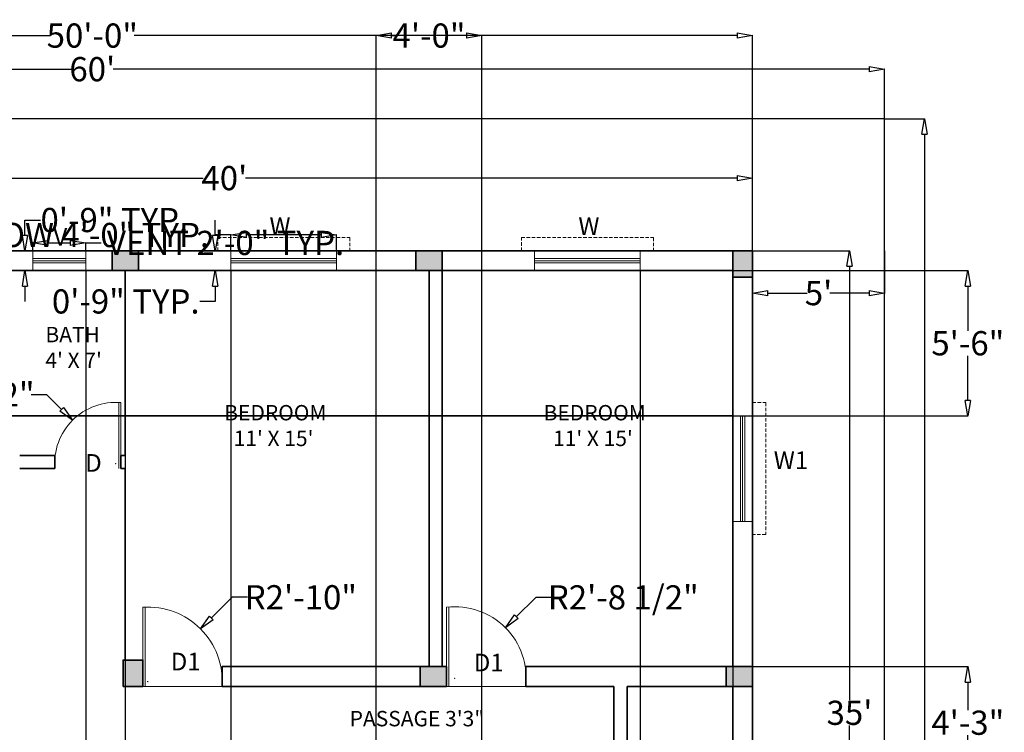
# Model space of a CAD drawing. Units: inches. Extents: x 668 to 1552, y 994 to 1684.
# Tile 4 of 4: x 1061 to 1509, y 1360 to 1684. Entities that reach past the tile are written whole.
import ezdxf

# ---------------------------------------------------------------- set-up
doc = ezdxf.new("R2010")
doc.units = ezdxf.units.IN
doc.header["$LTSCALE"] = 2.5
doc.header["$MEASUREMENT"] = 0
doc.linetypes.add('HIDDEN', pattern=[0.375, 0.25, -0.125])
for name, color, linetype, lineweight, true_color in [('A-ANNO-DIMS', 175, 'Continuous', 13, 0x4554a5), ('A-ANNO-TEXT', 52, 'Continuous', 18, 0xc8c92d), ('A-DOOR', 152, 'Continuous', 18, 0x2776bb)]:
    doc.layers.add(name, color=color, linetype=linetype, lineweight=lineweight, true_color=true_color)
for name, color, linetype, lineweight in [('A-AREA-IDEN', 2, 'Continuous', 18), ('A-COLS', 7, 'Continuous', 35), ('A-COLS-PATT', 1, 'Continuous', 13), ('A-GLAZ', 4, 'Continuous', 18), ('A-WALL', 7, 'Continuous', 35), ('C-PROP', 1, 'Continuous', 25), ('sajjas', 210, 'HIDDEN', 13)]:
    doc.layers.add(name, color=color, linetype=linetype, lineweight=lineweight)
doc.styles.get("Standard").update_dxf_attribs({"font": 'arial.ttf'})
doc.dimstyles.get("Standard").update_dxf_attribs({"dimtxt": 11, "dimasz": 7, "dimexe": 0.18, "dimexo": 0.0625, "dimgap": 0.09, "dimtad": 0, "dimtih": 1, "dimtoh": 1, "dimdec": 0, "dimzin": 0, "dimdsep": 46, "dimlunit": 3, "dimtxsty": 'Standard', "dimblk": 'CLOSEDBLANK', "dimcen": 0.09, "dimadec": 0, "dimazin": 0, "dimtfac": 1, "dimtdec": 0, "dimtofl": 0, "dimtmove": 0, "dimatfit": 3, "dimldrblk": 'CLOSEDBLANK', "dimfxl": 1, "dimtolj": 1, "dimtzin": 0, "dimarcsym": 0})

# ---------------------------------------------------------------- blocks, each defined once
blk = doc.blocks.new('_ClosedBlank')
at = {"color": 0, "linetype": 'ByBlock', "lineweight": -2}
for p, q in [((-1, 0.167), (0, 0)), ((-1, 0.167), (-1, -0.167)), ((0, 0), (-1, -0.167))]:
    blk.add_line(p, q, dxfattribs=at)
blk = doc.blocks.new('*D1')
at = {"layer": 'A-ANNO-DIMS', "color": 0, "lineweight": -2, "ltscale": 2.5, "transparency": 16777216}
for p, q in [((734.36, 1639.41), (734.36, 1662.1)), ((741.36, 1661.92), (1084.91, 1661.92)), ((1447.36, 1661.92), (1103.82, 1661.92)), ((1454.36, 1639.41), (1454.36, 1662.1))]:
    blk.add_line(p, q, dxfattribs=at)
at = {"layer": 'Defpoints', "color": 0, "ltscale": 2.5, "transparency": 16777216}
for p in [(1454.36, 1661.92), (734.36, 1639.35), (1454.36, 1639.35)]:
    blk.add_point(p, dxfattribs=at)
at = {"layer": 'A-ANNO-DIMS', "color": 0, "lineweight": -2, "ltscale": 2.5, "transparency": 16777216, "xscale": 7, "yscale": 7, "zscale": 7, "rotation": 180}
blk.add_blockref('_ClosedBlank', (734.36, 1661.92), dxfattribs=at)
at = {"layer": 'A-ANNO-DIMS', "color": 0, "lineweight": -2, "ltscale": 2.5, "transparency": 16777216, "xscale": 7, "yscale": 7, "zscale": 7}
blk.add_blockref('_ClosedBlank', (1454.36, 1661.92), dxfattribs=at)
at = {"layer": 'A-ANNO-DIMS', "color": 0, "ltscale": 2.5, "transparency": 16777216, "insert": (1094.36, 1661.92), "char_height": 11, "attachment_point": 5}
blk.add_mtext("\\A1;60'", dxfattribs=at)
blk = doc.blocks.new('*D2')
at = {"layer": 'A-ANNO-DIMS', "color": 0, "lineweight": -2, "ltscale": 2.5, "transparency": 16777216}
for p, q in [((1454.43, 1639.35), (1472.67, 1639.35)), ((1472.49, 1632.35), (1472.49, 1345.06)), ((1472.49, 1046.35), (1472.49, 1333.64)), ((1454.43, 1039.35), (1472.67, 1039.35))]:
    blk.add_line(p, q, dxfattribs=at)
at = {"layer": 'Defpoints', "color": 0, "ltscale": 2.5, "transparency": 16777216}
for p in [(1454.36, 1639.35), (1454.36, 1039.35), (1472.49, 1039.35)]:
    blk.add_point(p, dxfattribs=at)
at = {"layer": 'A-ANNO-DIMS', "color": 0, "lineweight": -2, "ltscale": 2.5, "transparency": 16777216, "xscale": 7, "yscale": 7, "zscale": 7}
for p, rotation in [((1472.49, 1639.35), 90), ((1472.49, 1039.35), 270)]:
    blk.add_blockref('_ClosedBlank', p, dxfattribs=dict(at, rotation=rotation))
at = {"layer": 'A-ANNO-DIMS', "color": 0, "ltscale": 2.5, "transparency": 16777216, "insert": (1472.49, 1339.35), "char_height": 11, "attachment_point": 5}
blk.add_mtext("\\A1;50'", dxfattribs=at)
blk = doc.blocks.new('*D3')
at = {"layer": 'A-ANNO-DIMS', "color": 0, "lineweight": -2, "ltscale": 2.5, "transparency": 16777216}
for p, q in [((914.36, 1579.41), (914.36, 1612.58)), ((921.36, 1612.4), (1144.72, 1612.4)), ((1387.36, 1612.4), (1164.01, 1612.4)), ((1394.36, 1579.41), (1394.36, 1612.58))]:
    blk.add_line(p, q, dxfattribs=at)
at = {"layer": 'Defpoints', "color": 0, "ltscale": 2.5, "transparency": 16777216}
for p in [(914.36, 1612.4), (914.36, 1579.35), (1394.36, 1579.35)]:
    blk.add_point(p, dxfattribs=at)
at = {"layer": 'A-ANNO-DIMS', "color": 0, "lineweight": -2, "ltscale": 2.5, "transparency": 16777216, "xscale": 7, "yscale": 7, "zscale": 7, "rotation": 180}
blk.add_blockref('_ClosedBlank', (914.36, 1612.4), dxfattribs=at)
at = {"layer": 'A-ANNO-DIMS', "color": 0, "lineweight": -2, "ltscale": 2.5, "transparency": 16777216, "xscale": 7, "yscale": 7, "zscale": 7}
blk.add_blockref('_ClosedBlank', (1394.36, 1612.4), dxfattribs=at)
at = {"layer": 'A-ANNO-DIMS', "color": 0, "ltscale": 2.5, "transparency": 16777216, "insert": (1154.36, 1612.4), "char_height": 11, "attachment_point": 5}
blk.add_mtext("\\A1;40'", dxfattribs=at)
blk = doc.blocks.new('*D8')
at = {"layer": 'A-ANNO-DIMS', "color": 0, "lineweight": -2, "ltscale": 2.5, "transparency": 16777216}
for p, q in [((1394.36, 1579.29), (1394.36, 1559.95)), ((1454.36, 1579.29), (1454.36, 1559.95)), ((1401.36, 1560.13), (1419.21, 1560.13)), ((1447.36, 1560.13), (1429.51, 1560.13))]:
    blk.add_line(p, q, dxfattribs=at)
at = {"layer": 'Defpoints', "color": 0, "ltscale": 2.5, "transparency": 16777216}
for p in [(1394.36, 1579.35), (1454.36, 1579.35), (1454.36, 1560.13)]:
    blk.add_point(p, dxfattribs=at)
at = {"layer": 'A-ANNO-DIMS', "color": 0, "lineweight": -2, "ltscale": 2.5, "transparency": 16777216, "xscale": 7, "yscale": 7, "zscale": 7, "rotation": 180}
blk.add_blockref('_ClosedBlank', (1394.36, 1560.13), dxfattribs=at)
at = {"layer": 'A-ANNO-DIMS', "color": 0, "lineweight": -2, "ltscale": 2.5, "transparency": 16777216, "xscale": 7, "yscale": 7, "zscale": 7}
blk.add_blockref('_ClosedBlank', (1454.36, 1560.13), dxfattribs=at)
at = {"layer": 'A-ANNO-DIMS', "color": 0, "ltscale": 2.5, "transparency": 16777216, "insert": (1424.36, 1560.13), "char_height": 11, "attachment_point": 5}
blk.add_mtext("\\A1;5'", dxfattribs=at)
blk = doc.blocks.new('*D9')
at = {"layer": 'A-ANNO-DIMS', "color": 0, "lineweight": -2, "ltscale": 2.5, "transparency": 16777216}
for p, q in [((1394.43, 1579.35), (1438.61, 1579.35)), ((1438.43, 1572.35), (1438.43, 1375.06)), ((1438.43, 1166.35), (1438.43, 1363.64)), ((1394.43, 1159.35), (1438.61, 1159.35))]:
    blk.add_line(p, q, dxfattribs=at)
at = {"layer": 'Defpoints', "color": 0, "ltscale": 2.5, "transparency": 16777216}
for p in [(1394.36, 1579.35), (1394.36, 1159.35), (1438.43, 1159.35)]:
    blk.add_point(p, dxfattribs=at)
at = {"layer": 'A-ANNO-DIMS', "color": 0, "lineweight": -2, "ltscale": 2.5, "transparency": 16777216, "xscale": 7, "yscale": 7, "zscale": 7}
for p, rotation in [((1438.43, 1579.35), 90), ((1438.43, 1159.35), 270)]:
    blk.add_blockref('_ClosedBlank', p, dxfattribs=dict(at, rotation=rotation))
at = {"layer": 'A-ANNO-DIMS', "color": 0, "ltscale": 2.5, "transparency": 16777216, "insert": (1438.43, 1369.35), "char_height": 11, "attachment_point": 5}
blk.add_mtext("\\A1;35'", dxfattribs=at)
blk = doc.blocks.new('WIN-48')
for p, q in [((0, 9), (48, 9)), ((0, 9), (0, 0)), ((48, 9), (48, 0)), ((48, 5.5), (0, 5.5)), ((48, 4.5), (0, 4.5)), ((48, 3.5), (0, 3.5)), ((0, 0), (48, 0))]:
    blk.add_line(p, q)
blk = doc.blocks.new('VENT-24')
for p, q in [((0, 9), (24, 9)), ((0, 0), (0, 9)), ((24, 9), (24, 0)), ((24, 5.5), (0.04, 5.5)), ((24, 4.5), (0.04, 4.5)), ((24, 0), (0, 0)), ((24, 3.5), (0.04, 3.5))]:
    blk.add_line(p, q)
blk = doc.blocks.new('SAJJA-60')
at = {"ltscale": 2.5}
blk.add_lwpolyline([(6, 6), (0, 6), (0, 0), (54, 0), (60, 0), (60, 6), (54, 6)], dxfattribs=at)
blk = doc.blocks.new('*D22')
at = {"layer": 'A-ANNO-DIMS', "color": 0, "lineweight": -2, "ltscale": 2.5, "transparency": 16777216}
for p, q in [((1157.36, 1586.55), (1150.36, 1586.55)), ((1157.36, 1579.41), (1157.36, 1586.73)), ((1198.36, 1586.55), (1164.36, 1586.55)), ((1205.36, 1579.41), (1205.36, 1586.73))]:
    blk.add_line(p, q, dxfattribs=at)
at = {"layer": 'Defpoints', "color": 0, "ltscale": 2.5, "transparency": 16777216}
for p in [(1157.36, 1586.55), (1157.36, 1579.35), (1205.36, 1579.35)]:
    blk.add_point(p, dxfattribs=at)
at = {"layer": 'A-ANNO-DIMS', "color": 0, "lineweight": -2, "ltscale": 2.5, "transparency": 16777216, "xscale": 7, "yscale": 7, "zscale": 7, "rotation": 180}
blk.add_blockref('_ClosedBlank', (1157.36, 1586.55), dxfattribs=at)
at = {"layer": 'A-ANNO-DIMS', "color": 0, "lineweight": -2, "ltscale": 2.5, "transparency": 16777216, "xscale": 7, "yscale": 7, "zscale": 7}
blk.add_blockref('_ClosedBlank', (1205.36, 1586.55), dxfattribs=at)
at = {"layer": 'A-ANNO-DIMS', "color": 0, "ltscale": 2.5, "transparency": 16777216, "insert": (1080.67, 1586.55), "char_height": 11, "attachment_point": 5}
blk.add_mtext('\\A1;WINDOW 4\'-0" TYP.', dxfattribs=at)
blk = doc.blocks.new('*D23')
at = {"layer": 'A-ANNO-DIMS', "color": 0, "lineweight": -2, "ltscale": 2.5, "transparency": 16777216}
for p, q in [((1150.16, 1586.35), (1150.16, 1593.35)), ((1157.3, 1579.35), (1149.98, 1579.35)), ((1157.3, 1570.35), (1149.98, 1570.35)), ((1150.16, 1563.35), (1150.16, 1556.35)), ((1150.16, 1556.35), (1143.16, 1556.35))]:
    blk.add_line(p, q, dxfattribs=at)
at = {"layer": 'Defpoints', "color": 0, "ltscale": 2.5, "transparency": 16777216}
for p in [(1157.36, 1579.35), (1150.16, 1570.35), (1157.36, 1570.35)]:
    blk.add_point(p, dxfattribs=at)
at = {"layer": 'A-ANNO-DIMS', "color": 0, "lineweight": -2, "ltscale": 2.5, "transparency": 16777216, "xscale": 7, "yscale": 7, "zscale": 7}
for p, rotation in [((1150.16, 1579.35), 270), ((1150.16, 1570.35), 90)]:
    blk.add_blockref('_ClosedBlank', p, dxfattribs=dict(at, rotation=rotation))
at = {"layer": 'A-ANNO-DIMS', "color": 0, "ltscale": 2.5, "transparency": 16777216, "insert": (1109.55, 1556.35), "char_height": 11, "attachment_point": 5}
blk.add_mtext('\\A1;0\'-9" TYP.', dxfattribs=at)
blk = doc.blocks.new('*D26')
at = {"layer": 'A-ANNO-DIMS', "color": 0, "lineweight": -2, "ltscale": 2.5, "transparency": 16777216}
for p, q in [((1067.36, 1579.41), (1067.36, 1583.13)), ((1074.36, 1582.95), (1084.36, 1582.95)), ((1091.36, 1579.41), (1091.36, 1583.13)), ((1091.36, 1582.95), (1098.36, 1582.95))]:
    blk.add_line(p, q, dxfattribs=at)
at = {"layer": 'Defpoints', "color": 0, "ltscale": 2.5, "transparency": 16777216}
for p in [(1091.36, 1582.95), (1067.36, 1579.35), (1091.36, 1579.35)]:
    blk.add_point(p, dxfattribs=at)
at = {"layer": 'A-ANNO-DIMS', "color": 0, "lineweight": -2, "ltscale": 2.5, "transparency": 16777216, "xscale": 7, "yscale": 7, "zscale": 7, "rotation": 180}
blk.add_blockref('_ClosedBlank', (1067.36, 1582.95), dxfattribs=at)
at = {"layer": 'A-ANNO-DIMS', "color": 0, "lineweight": -2, "ltscale": 2.5, "transparency": 16777216, "xscale": 7, "yscale": 7, "zscale": 7}
blk.add_blockref('_ClosedBlank', (1091.36, 1582.95), dxfattribs=at)
at = {"layer": 'A-ANNO-DIMS', "color": 0, "ltscale": 2.5, "transparency": 16777216, "insert": (1154.89, 1582.95), "char_height": 11, "attachment_point": 5}
blk.add_mtext('\\A1;VENT 2\'-0" TYP.', dxfattribs=at)
blk = doc.blocks.new('*D27')
at = {"layer": 'A-ANNO-DIMS', "color": 0, "lineweight": -2, "ltscale": 2.5, "transparency": 16777216}
for p, q in [((1063.76, 1586.35), (1063.76, 1593.35)), ((1063.76, 1593.35), (1070.76, 1593.35)), ((1067.3, 1579.35), (1063.58, 1579.35)), ((1067.3, 1570.35), (1063.58, 1570.35)), ((1063.76, 1563.35), (1063.76, 1556.35))]:
    blk.add_line(p, q, dxfattribs=at)
at = {"layer": 'Defpoints', "color": 0, "ltscale": 2.5, "transparency": 16777216}
for p in [(1063.76, 1579.35), (1067.36, 1579.35), (1067.36, 1570.35)]:
    blk.add_point(p, dxfattribs=at)
at = {"layer": 'A-ANNO-DIMS', "color": 0, "lineweight": -2, "ltscale": 2.5, "transparency": 16777216, "xscale": 7, "yscale": 7, "zscale": 7}
for p, rotation in [((1063.76, 1579.35), 270), ((1063.76, 1570.35), 90)]:
    blk.add_blockref('_ClosedBlank', p, dxfattribs=dict(at, rotation=rotation))
at = {"layer": 'A-ANNO-DIMS', "color": 0, "ltscale": 2.5, "transparency": 16777216, "insert": (1104.38, 1593.35), "char_height": 11, "attachment_point": 5}
blk.add_mtext('\\A1;0\'-9" TYP.', dxfattribs=at)
blk = doc.blocks.new('*D34')
at = {"layer": 'A-ANNO-DIMS', "color": 0, "lineweight": -2, "ltscale": 2.5, "transparency": 16777216}
for p, q in [((794.36, 1390.41), (794.36, 1677.38)), ((801.36, 1677.2), (1075.38, 1677.2)), ((1387.36, 1677.2), (1113.35, 1677.2)), ((1394.36, 1579.41), (1394.36, 1677.38))]:
    blk.add_line(p, q, dxfattribs=at)
at = {"layer": 'Defpoints', "color": 0, "ltscale": 2.5, "transparency": 16777216}
for p in [(1394.36, 1677.2), (1394.36, 1579.35), (794.36, 1390.35)]:
    blk.add_point(p, dxfattribs=at)
at = {"layer": 'A-ANNO-DIMS', "color": 0, "lineweight": -2, "ltscale": 2.5, "transparency": 16777216, "xscale": 7, "yscale": 7, "zscale": 7, "rotation": 180}
blk.add_blockref('_ClosedBlank', (794.36, 1677.2), dxfattribs=at)
at = {"layer": 'A-ANNO-DIMS', "color": 0, "lineweight": -2, "ltscale": 2.5, "transparency": 16777216, "xscale": 7, "yscale": 7, "zscale": 7}
blk.add_blockref('_ClosedBlank', (1394.36, 1677.2), dxfattribs=at)
at = {"layer": 'A-ANNO-DIMS', "color": 0, "ltscale": 2.5, "transparency": 16777216, "insert": (1094.36, 1677.2), "char_height": 11, "attachment_point": 5}
blk.add_mtext('\\A1;50\'-0"', dxfattribs=at)
blk = doc.blocks.new('*D39')
at = {"layer": 'A-ANNO-DIMS', "color": 0, "lineweight": -2, "ltscale": 2.5, "transparency": 16777216}
for p, q in [((1091.36, 1570.29), (1091.36, 1001.32)), ((1109.36, 1570.29), (1109.36, 1001.32)), ((1098.36, 1001.5), (1102.36, 1001.5)), ((1109.36, 1001.5), (1116.36, 1001.5))]:
    blk.add_line(p, q, dxfattribs=at)
at = {"layer": 'Defpoints', "color": 0, "ltscale": 2.5, "transparency": 16777216}
for p in [(1091.36, 1570.35), (1109.36, 1570.35), (1109.36, 1001.5)]:
    blk.add_point(p, dxfattribs=at)
at = {"layer": 'A-ANNO-DIMS', "color": 0, "lineweight": -2, "ltscale": 2.5, "transparency": 16777216, "xscale": 7, "yscale": 7, "zscale": 7, "rotation": 180}
blk.add_blockref('_ClosedBlank', (1091.36, 1001.5), dxfattribs=at)
at = {"layer": 'A-ANNO-DIMS', "color": 0, "lineweight": -2, "ltscale": 2.5, "transparency": 16777216, "xscale": 7, "yscale": 7, "zscale": 7}
blk.add_blockref('_ClosedBlank', (1109.36, 1001.5), dxfattribs=at)
at = {"layer": 'A-ANNO-DIMS', "color": 0, "ltscale": 2.5, "transparency": 16777216, "insert": (1130.56, 1001.5), "char_height": 11, "attachment_point": 5}
blk.add_mtext('\\A1;1\'-6"', dxfattribs=at)
blk = doc.blocks.new('*D40')
at = {"layer": 'A-ANNO-DIMS', "color": 0, "lineweight": -2, "ltscale": 2.5, "transparency": 16777216}
for p, q in [((1109.36, 1570.29), (1109.36, 1001.32)), ((1157.36, 1570.29), (1157.36, 1001.32)), ((1116.36, 1001.5), (1118.43, 1001.5)), ((1150.36, 1001.5), (1148.29, 1001.5))]:
    blk.add_line(p, q, dxfattribs=at)
at = {"layer": 'Defpoints', "color": 0, "ltscale": 2.5, "transparency": 16777216}
for p in [(1109.36, 1570.35), (1157.36, 1570.35), (1157.36, 1001.5)]:
    blk.add_point(p, dxfattribs=at)
at = {"layer": 'A-ANNO-DIMS', "color": 0, "lineweight": -2, "ltscale": 2.5, "transparency": 16777216, "xscale": 7, "yscale": 7, "zscale": 7, "rotation": 180}
blk.add_blockref('_ClosedBlank', (1109.36, 1001.5), dxfattribs=at)
at = {"layer": 'A-ANNO-DIMS', "color": 0, "lineweight": -2, "ltscale": 2.5, "transparency": 16777216, "xscale": 7, "yscale": 7, "zscale": 7}
blk.add_blockref('_ClosedBlank', (1157.36, 1001.5), dxfattribs=at)
at = {"layer": 'A-ANNO-DIMS', "color": 0, "ltscale": 2.5, "transparency": 16777216, "insert": (1133.36, 1001.5), "char_height": 11, "attachment_point": 5}
blk.add_mtext('\\A1;4\'-0"', dxfattribs=at)
blk = doc.blocks.new('*D41')
at = {"layer": 'A-ANNO-DIMS', "color": 0, "lineweight": -2, "ltscale": 2.5, "transparency": 16777216}
for p, q in [((1343.362549, 1570.287512), (1343.362549, 1001.320012)), ((1385.362549, 1570.287512), (1385.362549, 1001.320012)), ((1336.362549, 1001.500012), (1329.362549, 1001.500012)), ((1392.362549, 1001.500012), (1399.362549, 1001.500012))]:
    blk.add_line(p, q, dxfattribs=at)
at = {"layer": 'Defpoints', "color": 0, "ltscale": 2.5, "transparency": 16777216}
for p in [(1343.362549, 1570.350012), (1385.362549, 1570.350012), (1385.362549, 1001.500012)]:
    blk.add_point(p, dxfattribs=at)
at = {"layer": 'A-ANNO-DIMS', "color": 0, "lineweight": -2, "ltscale": 2.5, "transparency": 16777216, "xscale": 7, "yscale": 7, "zscale": 7}
blk.add_blockref('_ClosedBlank', (1343.362549, 1001.500012), dxfattribs=at)
at = {"layer": 'A-ANNO-DIMS', "color": 0, "lineweight": -2, "ltscale": 2.5, "transparency": 16777216, "xscale": 7, "yscale": 7, "zscale": 7, "rotation": 180}
blk.add_blockref('_ClosedBlank', (1385.362549, 1001.500012), dxfattribs=at)
at = {"layer": 'A-ANNO-DIMS', "color": 0, "ltscale": 2.5, "transparency": 16777216, "insert": (1364.362549, 1001.500012), "char_height": 11, "attachment_point": 5}
blk.add_mtext('\\A1;3\'-6"', dxfattribs=at)
blk = doc.blocks.new('*D42')
at = {"layer": 'A-ANNO-DIMS', "color": 0, "lineweight": -2, "ltscale": 2.5, "transparency": 16777216}
for p, q in [((1385.3, 1570.35), (696.33, 1570.35)), ((696.51, 1563.35), (696.51, 1543.06)), ((696.51, 1511.35), (696.51, 1531.64)), ((1385.3, 1504.35), (696.33, 1504.35))]:
    blk.add_line(p, q, dxfattribs=at)
at = {"layer": 'Defpoints', "color": 0, "ltscale": 2.5, "transparency": 16777216}
for p in [(1385.36, 1570.35), (696.51, 1504.35), (1385.36, 1504.35)]:
    blk.add_point(p, dxfattribs=at)
at = {"layer": 'A-ANNO-DIMS', "color": 0, "lineweight": -2, "ltscale": 2.5, "transparency": 16777216, "xscale": 7, "yscale": 7, "zscale": 7}
for p, rotation in [((696.51, 1570.35), 90), ((696.51, 1504.35), 270)]:
    blk.add_blockref('_ClosedBlank', p, dxfattribs=dict(at, rotation=rotation))
at = {"layer": 'A-ANNO-DIMS', "color": 0, "ltscale": 2.5, "transparency": 16777216, "insert": (696.51, 1537.35), "char_height": 11, "attachment_point": 5}
blk.add_mtext('\\A1;5\'-6"', dxfattribs=at)
blk = doc.blocks.new('*D43')
at = {"layer": 'A-ANNO-DIMS', "color": 0, "lineweight": -2, "ltscale": 2.5, "transparency": 16777216}
for p, q in [((923.43, 1570.35), (1492.39, 1570.35)), ((1492.21, 1563.35), (1492.21, 1543.06)), ((1492.21, 1511.35), (1492.21, 1531.64)), ((923.43, 1504.35), (1492.39, 1504.35))]:
    blk.add_line(p, q, dxfattribs=at)
at = {"layer": 'Defpoints', "color": 0, "ltscale": 2.5, "transparency": 16777216}
for p in [(923.36, 1570.35), (923.36, 1504.35), (1492.21, 1504.35)]:
    blk.add_point(p, dxfattribs=at)
at = {"layer": 'A-ANNO-DIMS', "color": 0, "lineweight": -2, "ltscale": 2.5, "transparency": 16777216, "xscale": 7, "yscale": 7, "zscale": 7}
for p, rotation in [((1492.21, 1570.35), 90), ((1492.21, 1504.35), 270)]:
    blk.add_blockref('_ClosedBlank', p, dxfattribs=dict(at, rotation=rotation))
at = {"layer": 'A-ANNO-DIMS', "color": 0, "ltscale": 2.5, "transparency": 16777216, "insert": (1492.21, 1537.35), "char_height": 11, "attachment_point": 5}
blk.add_mtext('\\A1;5\'-6"', dxfattribs=at)
blk = doc.blocks.new('*D49')
at = {"layer": 'A-ANNO-DIMS', "color": 0, "lineweight": -2, "ltscale": 2.5, "transparency": 16777216}
for p, q in [((1223.36, 1168.41), (1223.36, 1677.38)), ((1230.36, 1677.2), (1232.43, 1677.2)), ((1264.36, 1677.2), (1262.29, 1677.2)), ((1271.36, 1168.41), (1271.36, 1677.38))]:
    blk.add_line(p, q, dxfattribs=at)
at = {"layer": 'Defpoints', "color": 0, "ltscale": 2.5, "transparency": 16777216}
for p in [(1271.36, 1677.2), (1223.36, 1168.35), (1271.36, 1168.35)]:
    blk.add_point(p, dxfattribs=at)
at = {"layer": 'A-ANNO-DIMS', "color": 0, "lineweight": -2, "ltscale": 2.5, "transparency": 16777216, "xscale": 7, "yscale": 7, "zscale": 7, "rotation": 180}
blk.add_blockref('_ClosedBlank', (1223.36, 1677.2), dxfattribs=at)
at = {"layer": 'A-ANNO-DIMS', "color": 0, "lineweight": -2, "ltscale": 2.5, "transparency": 16777216, "xscale": 7, "yscale": 7, "zscale": 7}
blk.add_blockref('_ClosedBlank', (1271.36, 1677.2), dxfattribs=at)
at = {"layer": 'A-ANNO-DIMS', "color": 0, "ltscale": 2.5, "transparency": 16777216, "insert": (1247.36, 1677.2), "char_height": 11, "attachment_point": 5}
blk.add_mtext('\\A1;4\'-0"', dxfattribs=at)
blk = doc.blocks.new('*D50')
at = {"layer": 'A-ANNO-DIMS', "color": 0, "lineweight": -2, "ltscale": 2.5, "transparency": 16777216}
for p, q in [((1394.43, 1390.35), (1492.39, 1390.35)), ((1492.21, 1383.35), (1492.21, 1370.56)), ((1492.21, 1346.35), (1492.21, 1359.14)), ((1394.43, 1339.35), (1492.39, 1339.35))]:
    blk.add_line(p, q, dxfattribs=at)
at = {"layer": 'Defpoints', "color": 0, "ltscale": 2.5, "transparency": 16777216}
for p in [(1394.36, 1390.35), (1394.36, 1339.35), (1492.21, 1339.35)]:
    blk.add_point(p, dxfattribs=at)
at = {"layer": 'A-ANNO-DIMS', "color": 0, "lineweight": -2, "ltscale": 2.5, "transparency": 16777216, "xscale": 7, "yscale": 7, "zscale": 7}
for p, rotation in [((1492.21, 1390.35), 90), ((1492.21, 1339.35), 270)]:
    blk.add_blockref('_ClosedBlank', p, dxfattribs=dict(at, rotation=rotation))
at = {"layer": 'A-ANNO-DIMS', "color": 0, "ltscale": 2.5, "transparency": 16777216, "insert": (1492.21, 1364.85), "char_height": 11, "attachment_point": 5}
blk.add_mtext('\\A1;4\'-3"', dxfattribs=at)
blk = doc.blocks.new('*D53')
at = {"layer": 'A-ANNO-DIMS', "color": 0, "lineweight": -2, "ltscale": 2.5, "transparency": 16777216}
for p, q in [((1157.88, 1421.87), (1148.48, 1412.47)), ((1164.88, 1421.87), (1157.88, 1421.87)), ((1119.53, 1383.6), (1119.71, 1383.6)), ((1119.62, 1383.51), (1119.62, 1383.69))]:
    blk.add_line(p, q, dxfattribs=at)
at = {"layer": 'Defpoints', "color": 0, "ltscale": 2.5, "transparency": 16777216}
for p in [(1143.53, 1407.52), (1119.62, 1383.6)]:
    blk.add_point(p, dxfattribs=at)
at = {"layer": 'A-ANNO-DIMS', "color": 0, "lineweight": -2, "ltscale": 2.5, "transparency": 16777216, "xscale": 7, "yscale": 7, "zscale": 7, "rotation": 224.9994441642691}
blk.add_blockref('_ClosedBlank', (1143.53, 1407.52), dxfattribs=at)
at = {"layer": 'A-ANNO-DIMS', "color": 0, "ltscale": 2.5, "transparency": 16777216, "insert": (1189.13, 1421.87), "char_height": 11, "attachment_point": 5}
blk.add_mtext('\\A1;R2\'-10"', dxfattribs=at)
blk = doc.blocks.new('*D57')
at = {"layer": 'A-ANNO-DIMS', "color": 0, "lineweight": -2, "ltscale": 2.5, "transparency": 16777216}
for p, q in [((1295.85, 1421.83), (1287, 1412.99)), ((1302.85, 1421.83), (1295.85, 1421.83)), ((1258.98, 1385.06), (1259.16, 1385.06)), ((1259.07, 1384.97), (1259.07, 1385.15))]:
    blk.add_line(p, q, dxfattribs=at)
at = {"layer": 'Defpoints', "color": 0, "ltscale": 2.5, "transparency": 16777216}
for p in [(1282.05, 1408.04), (1259.07, 1385.06)]:
    blk.add_point(p, dxfattribs=at)
at = {"layer": 'A-ANNO-DIMS', "color": 0, "lineweight": -2, "ltscale": 2.5, "transparency": 16777216, "xscale": 7, "yscale": 7, "zscale": 7, "rotation": 224.9994216860455}
blk.add_blockref('_ClosedBlank', (1282.05, 1408.04), dxfattribs=at)
at = {"layer": 'A-ANNO-DIMS', "color": 0, "ltscale": 2.5, "transparency": 16777216, "insert": (1335.64, 1421.83), "char_height": 11, "attachment_point": 5}
blk.add_mtext('\\A1;R2\'-8 1/2"', dxfattribs=at)
blk = doc.blocks.new('*D59')
at = {"layer": 'A-ANNO-DIMS', "color": 0, "lineweight": -2, "ltscale": 2.5, "transparency": 16777216}
for p, q in [((1066.62, 1514.09), (1073.62, 1514.09)), ((1073.62, 1514.09), (1080.43, 1507.28)), ((1104.9, 1482.72), (1105.08, 1482.72)), ((1104.99, 1482.63), (1104.99, 1482.81))]:
    blk.add_line(p, q, dxfattribs=at)
at = {"layer": 'Defpoints', "color": 0, "ltscale": 2.5, "transparency": 16777216}
for p in [(1085.38, 1502.33), (1104.99, 1482.72)]:
    blk.add_point(p, dxfattribs=at)
at = {"layer": 'A-ANNO-DIMS', "color": 0, "lineweight": -2, "ltscale": 2.5, "transparency": 16777216, "xscale": 7, "yscale": 7, "zscale": 7, "rotation": 315.0008195408938}
blk.add_blockref('_ClosedBlank', (1085.38, 1502.33), dxfattribs=at)
at = {"layer": 'A-ANNO-DIMS', "color": 0, "ltscale": 2.5, "transparency": 16777216, "insert": (1033.83, 1514.09), "char_height": 11, "attachment_point": 5}
blk.add_mtext('\\A1;R2\'-3 1/2"', dxfattribs=at)

msp = doc.modelspace()

# ---------------------------------------------------------------- hatches: boundary and pattern name
at = {"layer": 'A-COLS-PATT'}
h = msp.add_hatch(color=256, dxfattribs=at)
h.dxf.hatch_style = 1
h.paths.add_polyline_path([(803.36, 1390.35), (794.36, 1390.35), (794.36, 1378.35), (803.36, 1378.35)])
h.paths.add_polyline_path([(1117.36, 1393.35), (1108.36, 1393.35), (1108.36, 1381.35), (1117.36, 1381.35)])
h.paths.add_polyline_path([(1255.36, 1390.35), (1243.36, 1390.35), (1243.36, 1381.35), (1255.36, 1381.35)])
h.paths.add_polyline_path([(1394.36, 1390.35), (1382.36, 1390.35), (1382.36, 1381.35), (1394.36, 1381.35)])
h.paths.add_polyline_path([(1394.36, 1579.35), (1385.36, 1579.35), (1385.36, 1567.35), (1394.36, 1567.35)])
h.paths.add_polyline_path([(1253.36, 1579.35), (1241.36, 1579.35), (1241.36, 1570.35), (1253.36, 1570.35)])
h.paths.add_polyline_path([(1115.36, 1579.35), (1103.36, 1579.35), (1103.36, 1570.35), (1115.36, 1570.35)])
h.paths.add_polyline_path([(923.36, 1579.35), (914.36, 1579.35), (914.36, 1567.35), (923.36, 1567.35)])
h.paths.add_polyline_path([(926.36, 1390.35), (914.36, 1390.35), (914.36, 1381.35), (926.36, 1381.35)])
h.paths.add_polyline_path([(1394.36, 1243.35), (1382.36, 1243.35), (1382.36, 1234.35), (1394.36, 1234.35)])
h.paths.add_polyline_path([(1277.36, 1342.35), (1265.36, 1342.35), (1265.36, 1333.35), (1277.36, 1333.35)])
h.paths.add_polyline_path([(1130.36, 1311.02), (1121.36, 1311.02), (1121.36, 1299.02), (1130.36, 1299.02)])
h.paths.add_polyline_path([(1043.36, 1311.02), (1034.36, 1311.02), (1034.36, 1299.02), (1043.36, 1299.02)])
h.paths.add_polyline_path([(803.36, 1171.35), (794.36, 1171.35), (794.36, 1159.35), (803.36, 1159.35)])
h.paths.add_polyline_path([(1046.36, 1168.35), (1034.36, 1168.35), (1034.36, 1159.35), (1046.36, 1159.35)])
h.paths.add_polyline_path([(1133.36, 1168.35), (1121.36, 1168.35), (1121.36, 1159.35), (1133.36, 1159.35)])
h.paths.add_polyline_path([(1277.36, 1168.35), (1265.36, 1168.35), (1265.36, 1159.35), (1277.36, 1159.35)])

# ---------------------------------------------------------------- linework, layer by layer
at = {"layer": 'A-COLS'}
for points in [[(1115.36, 1570.35), (1115.36, 1579.35), (1103.36, 1579.35), (1103.36, 1570.35)], [(1253.36, 1570.35), (1253.36, 1579.35), (1241.36, 1579.35), (1241.36, 1570.35)], [(1385.36, 1567.35), (1394.36, 1567.35), (1394.36, 1579.35), (1385.36, 1579.35)], [(1108.36, 1381.35), (1117.36, 1381.35), (1117.36, 1393.35), (1108.36, 1393.35)], [(1255.36, 1381.35), (1255.36, 1390.35), (1243.36, 1390.35), (1243.36, 1381.35)], [(1394.36, 1381.35), (1394.36, 1390.35), (1382.36, 1390.35), (1382.36, 1381.35)]]:
    msp.add_lwpolyline(points, close=True, dxfattribs=at)
at = {"layer": 'A-DOOR'}
for p, q in [((1106.36, 1480.35), (1106.36, 1510.35)), ((1107.36, 1480.35), (1107.36, 1510.35)), ((1117.36, 1381.35), (1117.36, 1417.35)), ((1118.36, 1381.35), (1118.36, 1417.35)), ((1255.36, 1381.35), (1255.36, 1417.35)), ((1256.36, 1381.35), (1256.36, 1417.35)), ((1117.36, 1381.35), (1153.36, 1381.35)), ((1254.36, 1381.35), (1291.36, 1381.35))]:
    msp.add_line(p, q, dxfattribs=at)
for centre, radius, start, end in [((1104.99, 1482.72), 27.73, 85.1016, 184.8984), ((1119.62, 1383.6), 33.82, 356.1772, 93.8228), ((1259.07, 1385.06), 32.51, 353.4533, 96.5467)]:
    msp.add_arc(centre, radius, start, end, dxfattribs=at)
at = {"layer": 'A-GLAZ'}
for p, q in [((1067.36, 1570.35), (1067.36, 1579.35)), ((1091.36, 1570.35), (1091.36, 1579.35)), ((1157.36, 1570.35), (1157.36, 1579.35)), ((1205.36, 1570.35), (1205.36, 1579.35))]:
    msp.add_line(p, q, dxfattribs=at)
at = {"layer": 'A-WALL'}
for p, q in [((1394.36, 1579.35), (914.36, 1579.35)), ((1394.36, 1234.35), (1394.36, 1579.35)), ((1109.36, 1570.35), (1061.36, 1570.35)), ((1109.36, 1486.35), (1109.36, 1570.35)), ((1247.36, 1570.35), (1115.36, 1570.35)), ((1247.36, 1390.35), (1247.36, 1570.35)), ((1385.36, 1570.35), (1253.36, 1570.35)), ((1253.36, 1390.35), (1253.36, 1570.35)), ((1385.36, 1390.35), (1385.36, 1570.35)), ((1077.36, 1486.35), (1061.36, 1486.35)), ((1077.36, 1486.35), (1077.36, 1480.35)), ((1109.36, 1486.35), (1107.36, 1486.35)), ((1107.36, 1486.35), (1107.36, 1480.35)), ((1077.36, 1480.35), (1061.36, 1480.35)), ((1109.36, 1480.35), (1107.36, 1480.35)), ((1109.36, 1393.35), (1109.36, 1480.35)), ((1117.36, 1390.35), (1117.36, 1381.35)), ((1247.36, 1390.35), (1153.36, 1390.35)), ((1153.36, 1390.35), (1153.36, 1381.35)), ((1255.36, 1390.35), (1253.36, 1390.35)), ((1255.36, 1390.35), (1255.36, 1381.35)), ((1385.36, 1390.35), (1291.36, 1390.35)), ((1291.36, 1390.35), (1291.36, 1381.35)), ((1117.36, 1381.35), (1109.36, 1381.35)), ((1255.36, 1381.35), (1153.36, 1381.35)), ((1255.36, 1381.35), (1253.36, 1381.35)), ((1331.36, 1381.35), (1291.36, 1381.35)), ((1331.36, 1381.35), (1291.36, 1381.35)), ((1331.36, 1327.35), (1331.36, 1381.35)), ((1385.36, 1381.35), (1337.36, 1381.35)), ((1385.36, 1381.35), (1337.36, 1381.35)), ((1337.36, 1327.35), (1337.36, 1381.35)), ((1385.36, 1297.35), (1385.36, 1381.35))]:
    msp.add_line(p, q, dxfattribs=at)
at = {"layer": 'C-PROP', "ltscale": 2.5}
for p, q in [((1454.36, 1639.35), (734.36, 1639.35)), ((1454.36, 1039.35), (1454.36, 1639.35))]:
    msp.add_line(p, q, dxfattribs=at)

# ---------------------------------------------------------------- block references
at = {"layer": 'A-GLAZ'}
msp.add_blockref('VENT-24', (1067.36, 1570.35), dxfattribs=at)
for p, rotation in [((1205.36, 1579.35), 180), ((1343.36, 1579.35), 180), ((1385.36, 1504.35), 270.0000000000009)]:
    msp.add_blockref('WIN-48', p, dxfattribs=dict(at, rotation=rotation))
at = {"layer": 'sajjas', "extrusion": (0, 0, -1), "zscale": -1}
for p, rotation in [((-1151.36, 1585.35), 180), ((-1289.36, 1585.35), 180), ((-1400.36, 1510.35), 270.0000000000003)]:
    msp.add_blockref('SAJJA-60', p, dxfattribs=dict(at, rotation=rotation))

# ---------------------------------------------------------------- texts
at = {"layer": 'A-ANNO-TEXT', "ltscale": 2.5, "char_height": 8, "attachment_point": 1}
for s, insert in [('W', (1174.86, 1594.63)), ('W', (1315.23, 1594.59)), ('V', (1076.67, 1589.68)), ('D', (1091.12, 1486.95)), ('W1', (1404.01, 1488.17)), ('D1', (1130.02, 1396.65)), ('D1', (1267.72, 1396.19))]:
    msp.add_mtext_dynamic_manual_height_columns(s, width=96.0512, gutter_width=1, heights=[0], dxfattribs=dict(at, insert=insert))
at = {"layer": 'A-AREA-IDEN', "ltscale": 2.5, "char_height": 7, "attachment_point": 1}
for s, width, insert in [("BATH\\P4' X 7'", 47.3322, (1073.04, 1544.79)), ("BEDROOM\\P  11' X 15'", 47.3322, (1154.31, 1509.27)), ("BEDROOM\\P  11' X 15'", 47.3322, (1299.43, 1509.27)), ('PASSAGE 3\'3"', 90.3192, (1211.3, 1370.21))]:
    msp.add_mtext_dynamic_manual_height_columns(s, width=width, gutter_width=1, heights=[0], dxfattribs=dict(at, insert=insert))

# ---------------------------------------------------------------- dimensions: what is measured, and where the dimension line sits
at = {"layer": 'A-ANNO-DIMS', "ltscale": 2.5}
for base, p1, p2, override, picture, middle in [((1394.36, 1677.2), (794.36, 1390.35), (1394.36, 1579.35), {"dimdec": 1, "dimlfac": 1, "dimrnd": 0, "dimzin": 1, "dimdsep": 46, "dimlunit": 4, "dimfrac": 2}, '*D34', (1094.36, 1677.2)), ((1271.36, 1677.2), (1223.36, 1168.35), (1271.36, 1168.35), {"dimdec": 1, "dimlfac": 1, "dimrnd": 0, "dimzin": 1, "dimdsep": 46, "dimlunit": 4, "dimfrac": 2}, '*D49', (1247.36, 1677.2)), ((1454.36, 1661.92), (734.36, 1639.35), (1454.36, 1639.35), {"dimclrd": 0, "dimclre": 0, "dimclrt": 0}, '*D1', (1094.36, 1661.92)), ((914.36, 1612.4), (1394.36, 1579.35), (914.36, 1579.35), {"dimclrd": 0, "dimclre": 0, "dimclrt": 0}, '*D3', (1154.36, 1612.4)), ((1454.36, 1560.13), (1394.36, 1579.35), (1454.36, 1579.35), {"dimclrd": 0, "dimclre": 0, "dimclrt": 0}, '*D8', (1424.36, 1560.13)), ((1109.36, 1001.5), (1091.36, 1570.35), (1109.36, 1570.35), {"dimdec": 1, "dimlfac": 1, "dimrnd": 0, "dimzin": 1, "dimdsep": 46, "dimlunit": 4, "dimfrac": 2}, '*D39', (1130.56, 1001.5)), ((1157.36, 1001.5), (1109.36, 1570.35), (1157.36, 1570.35), {"dimdec": 1, "dimlfac": 1, "dimrnd": 0, "dimzin": 1, "dimdsep": 46, "dimlunit": 4, "dimfrac": 2}, '*D40', (1133.36, 1001.5)), ((1385.36, 1001.5), (1343.36, 1570.35), (1385.36, 1570.35), {"dimdec": 1, "dimlfac": 1, "dimrnd": 0, "dimzin": 1, "dimdsep": 46, "dimlunit": 4, "dimfrac": 2}, '*D41', (1364.36, 1001.5))]:
    dim = msp.add_linear_dim(base=base, p1=p1, p2=p2, dimstyle='Standard', override=override, dxfattribs=at)
    dim.commit()
    dim.dimension.update_dxf_attribs({"geometry": picture, "text_midpoint": middle})
for base, p1, p2, override, picture, middle in [((1472.49, 1039.35), (1454.36, 1639.35), (1454.36, 1039.35), {"dimclrd": 0, "dimclre": 0, "dimclrt": 0}, '*D2', (1472.49, 1339.35)), ((1438.43, 1159.35), (1394.36, 1579.35), (1394.36, 1159.35), {"dimclrd": 0, "dimclre": 0, "dimclrt": 0}, '*D9', (1438.43, 1369.35)), ((696.51, 1504.35), (1385.36, 1570.35), (1385.36, 1504.35), {"dimdec": 1, "dimlfac": 1, "dimrnd": 0, "dimzin": 1, "dimdsep": 46, "dimlunit": 4, "dimfrac": 2}, '*D42', (696.51, 1537.35)), ((1492.21, 1504.35), (923.36, 1570.35), (923.36, 1504.35), {"dimdec": 1, "dimlfac": 1, "dimrnd": 0, "dimzin": 1, "dimdsep": 46, "dimlunit": 4, "dimfrac": 2}, '*D43', (1492.21, 1537.35)), ((1492.21, 1339.35), (1394.36, 1390.35), (1394.36, 1339.35), {"dimdec": 1, "dimlfac": 1, "dimrnd": 0, "dimzin": 1, "dimdsep": 46, "dimlunit": 4, "dimfrac": 2}, '*D50', (1492.21, 1364.85))]:
    dim = msp.add_linear_dim(base=base, p1=p1, p2=p2, angle=90, dimstyle='Standard', override=override, dxfattribs=at)
    dim.commit()
    dim.dimension.update_dxf_attribs({"geometry": picture, "text_midpoint": middle})
for base, p1, p2, angle, text, picture, middle in [((1157.36, 1586.55), (1205.36, 1579.35), (1157.36, 1579.35), 180, 'WINDOW <> TYP.', '*D22', (1080.67, 1586.55)), ((1063.76, 1579.35), (1067.36, 1570.35), (1067.36, 1579.35), 90, '<> TYP.', '*D27', (1104.38, 1593.35)), ((1150.16, 1570.35), (1157.36, 1579.35), (1157.36, 1570.35), 270, '<> TYP.', '*D23', (1109.55, 1556.35))]:
    dim = msp.add_linear_dim(base=base, p1=p1, p2=p2, angle=angle, text=text, dimstyle='Standard', override={"dimdec": 1, "dimlfac": 1, "dimrnd": 0, "dimzin": 1, "dimdsep": 46, "dimlunit": 4, "dimfrac": 2}, dxfattribs=at)
    dim.commit()
    dim.dimension.update_dxf_attribs({"geometry": picture, "text_midpoint": middle})
dim = msp.add_linear_dim(base=(1091.36, 1582.95), p1=(1067.36, 1579.35), p2=(1091.36, 1579.35), text='VENT <> TYP.', dimstyle='Standard', override={"dimdec": 1, "dimlfac": 1, "dimrnd": 0, "dimzin": 1, "dimdsep": 46, "dimlunit": 4, "dimfrac": 2}, dxfattribs=at)
dim.commit()
dim.dimension.update_dxf_attribs({"geometry": '*D26', "text_midpoint": (1154.89, 1582.95)})
for center, mpoint, picture, middle in [((1104.99, 1482.72), (1085.38, 1502.33), '*D59', (1033.83, 1514.09)), ((1259.07, 1385.06), (1282.05, 1408.04), '*D57', (1335.64, 1421.83)), ((1119.62, 1383.6), (1143.53, 1407.52), '*D53', (1189.13, 1421.87))]:
    dim = msp.add_radius_dim(center=center, mpoint=mpoint, dimstyle='Standard', override={"dimdec": 1, "dimlfac": 1, "dimrnd": 0, "dimzin": 1, "dimdsep": 46, "dimlunit": 4, "dimfrac": 2}, dxfattribs=at)
    dim.commit()
    dim.dimension.update_dxf_attribs({"geometry": picture, "text_midpoint": middle, "dimtype": 164})

doc.saveas('drawing.dxf')
